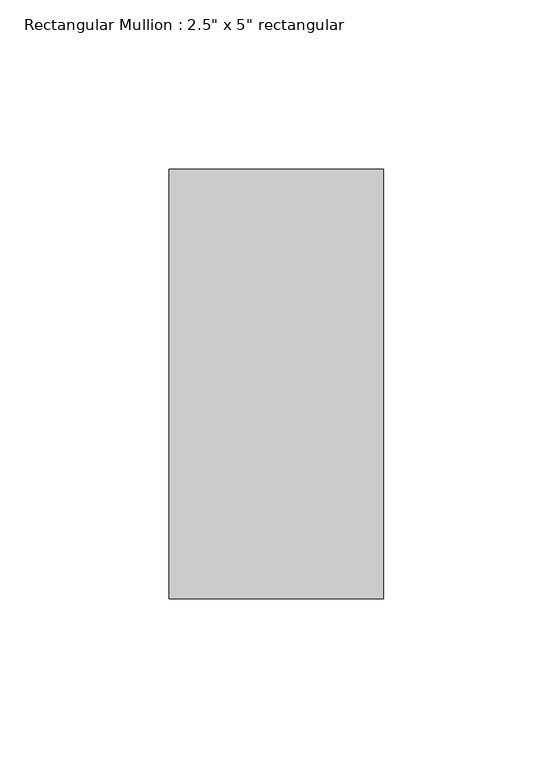
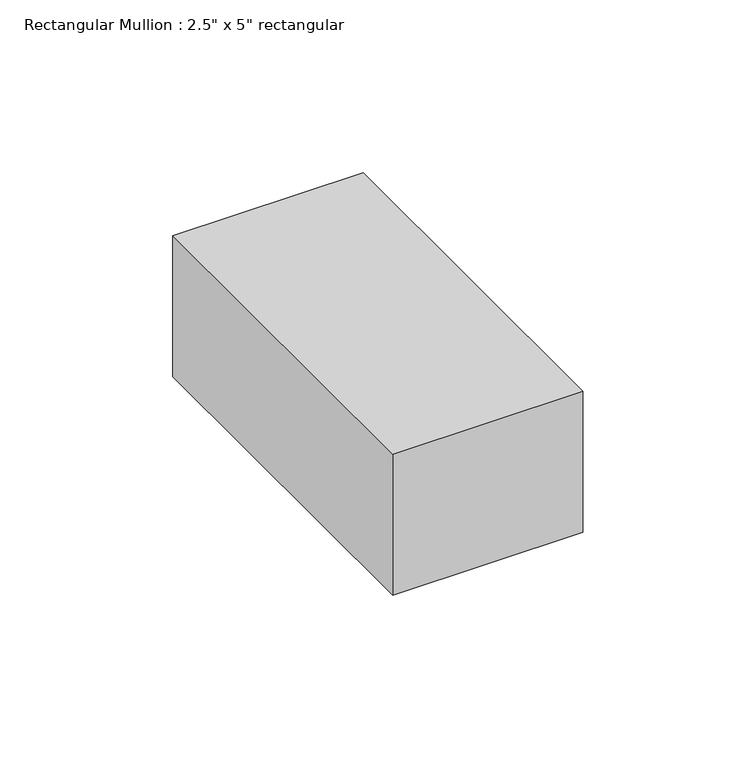
"""IFC4 building model written with IfcOpenShell, lengths in millimetres: member geometry."""

from ifc_helpers import new_model, si_unit, frame, origin, place, context, project, spatial, polyline, outline, extrude, source, transform, mapped, element, save


def member_e0baf447(model_context):
    return source(origin(), model_context, "Body", "SweptSolid", [
        extrude(outline(polyline([(0.0, 63.5), (0.0, -63.5), (-63.5, -63.5), (-63.5, 63.5), (0.0, 63.5)])), frame((0.0, 0.0, -49.779075), z_axis=(0.0, 0.0, 1.0), x_axis=(1.0, 0.0, 0.0)), (0.0, 0.0, 1.0), 49.779075),
    ])


if __name__ == "__main__":
    model = new_model("IFC4")
    model_context = context("Model", 3, world=origin())
    ifc_project = project(units=[si_unit("LENGTHUNIT", "METRE", prefix="MILLI")], contexts=[model_context])
    site = spatial("IfcSite", under=ifc_project)
    building = spatial("IfcBuilding", under=site)
    placement = place(None, origin())
    member_shape = member_e0baf447(model_context)
    element("IfcMember", 1, ObjectType="Rectangular Mullion : 2.5\" x 5\" rectangular", at=placement, inside=building, context=model_context, shape_type="MappedRepresentation", body=[
        mapped(member_shape, transform((0.0, 0.0, 0.0), x_axis=(1.0, 0.0, 0.0), y_axis=(0.0, 1.0, 0.0), z_axis=(0.0, 0.0, 1.0))),
    ])
    save(model, "model.ifc")

# Revit data of these elements
# Type "Rectangular Mullion : 2.5\" x 5\" rectangular"
#   built-in parameter 1007304 = 0.416667 (stored number, unit not read)
#   built-in parameter 1007301 = 0.104167 (stored number, unit not read)
#   built-in parameter 1007300 = 0.104167 (stored number, unit not read)
# Element 1 (IfcMember, "Rectangular Mullion : 2.5\" x 5\" rectangular")
#   Materials on its faces: "BLACK MATERIAL"
# Materials
#   "BLACK MATERIAL": class "Generic", colour RGB 120 120 120, transparency 0, Cost = 0
